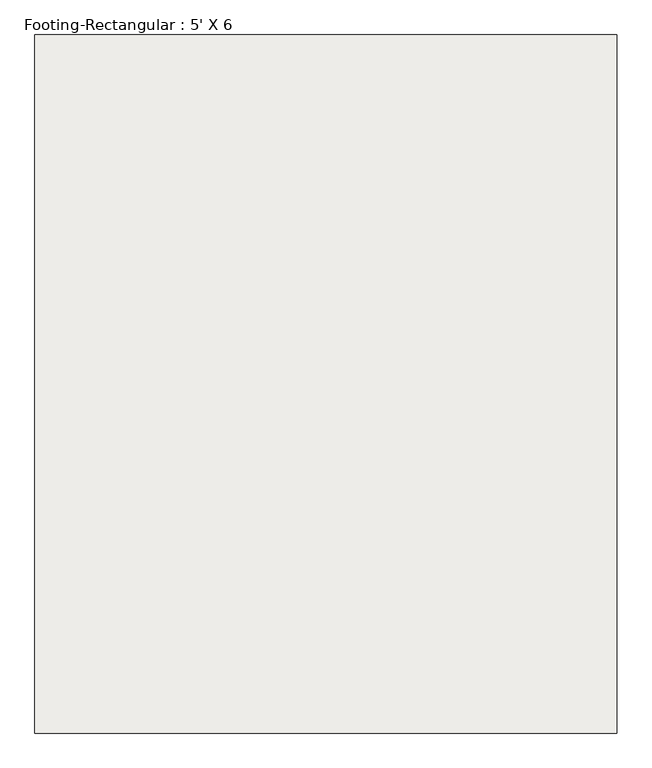
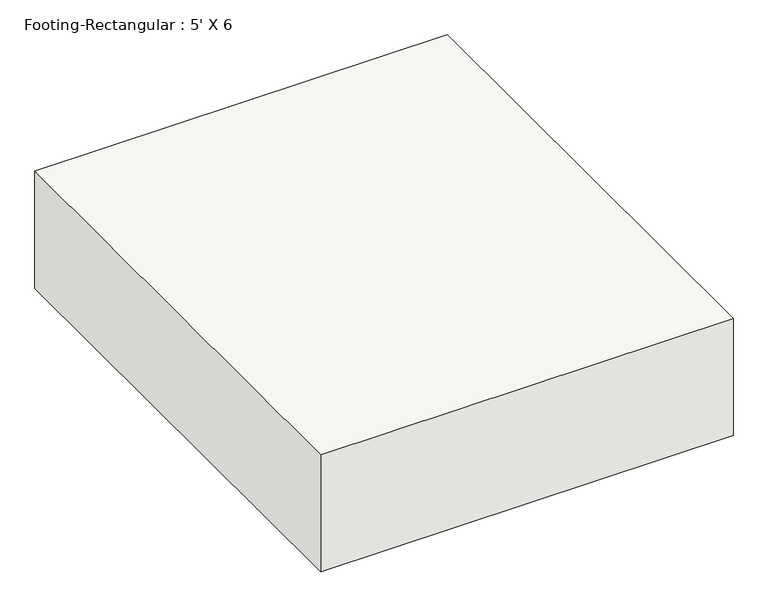
"""IFC4 building model written with IfcOpenShell, lengths in millimetres: slab geometry, Footing-Rectangular : 5' X 6."""

from ifc_helpers import new_model, si_unit, frame, origin, place, context, project, spatial, polyline, outline, extrude, source, transform, mapped, element, save


def footing_rectangular_5_x_6_26a6a031(model_context):
    return source(origin(), model_context, "Body", "SweptSolid", [
        extrude(outline(polyline([(762.0, 914.4), (762.0, -914.4), (-762.0, -914.4), (-762.0, 914.4), (762.0, 914.4)])), frame((0.0, 0.0, -457.2), z_axis=(0.0, 0.0, 1.0), x_axis=(1.0, 0.0, 0.0)), (0.0, 0.0, 1.0), 457.2),
    ])


if __name__ == "__main__":
    model = new_model("IFC4")
    model_context = context("Model", 3, world=origin())
    ifc_project = project(units=[si_unit("LENGTHUNIT", "METRE", prefix="MILLI")], contexts=[model_context])
    site = spatial("IfcSite", under=ifc_project)
    building = spatial("IfcBuilding", under=site)
    placement = place(None, origin())
    footing_rectangular_5_x_6_shape = footing_rectangular_5_x_6_26a6a031(model_context)
    element("IfcSlab", 1, ObjectType="Footing-Rectangular : 5' X 6", at=placement, inside=building, context=model_context, shape_type="MappedRepresentation", body=[
        mapped(footing_rectangular_5_x_6_shape, transform((0.0, 0.0, 0.0), x_axis=(1.0, 0.0, 0.0), y_axis=(0.0, 1.0, 0.0), z_axis=(0.0, 0.0, 1.0))),
    ])
    save(model, "model.ifc")

# Revit data of these elements
# Type "Footing-Rectangular : 5' X 6"
#   Assembly Code = "A1010100"
#   Width = 5' - 0"
#   Length = 6' - 0"
#   Foundation Thickness = 1' - 6"
#   Structural Material [instance default] = Concrete, Cast-in-Place gray
# Element 1 (IfcSlab, "Footing-Rectangular : 5' X 6")
#   Materials on its faces: "Concrete, Cast-in-Place gray"
# Materials
#   "Concrete, Cast-in-Place gray": class "Concrete", colour RGB 192 192 192, transparency 0, Description = "Cast-in-place concrete", Cost = 0
